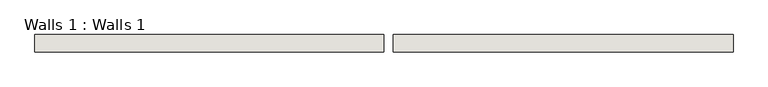
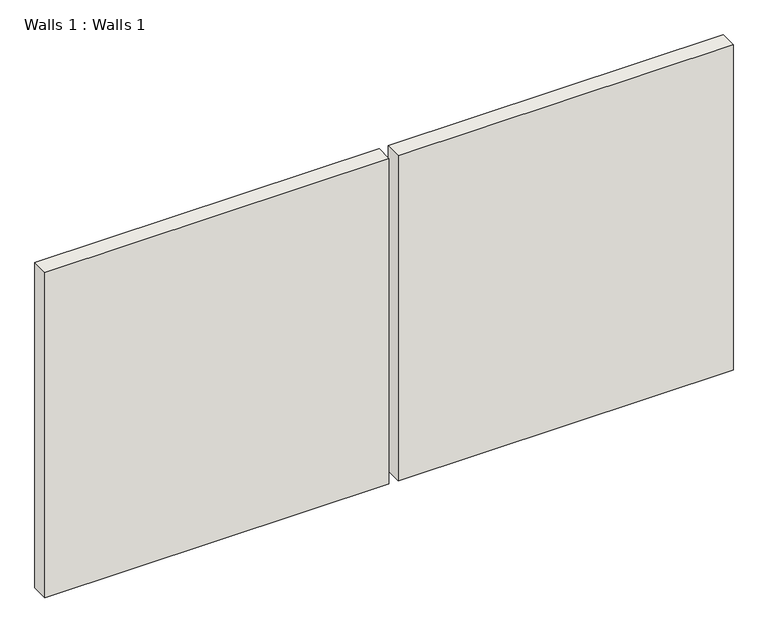
"""IFC4 building model written with IfcOpenShell, lengths in millimetres: wall geometry, Walls 1 : Walls 1."""

from ifc_helpers import new_model, si_unit, origin, origin_with_axes, place, context, project, spatial, polyline, outline, extrude, source, transform, mapped, element, save


def walls_1_walls_1_5f19503e(model_context):
    return source(origin(), model_context, "Body", "SweptSolid", [
        extrude(outline(polyline([(-9840.5692849, -1156.6793133), (-9840.5692849, -1080.4793133), (-8316.5692849, -1080.4793133), (-8316.5692849, -1156.6793133), (-9840.5692849, -1156.6793133)])), origin_with_axes(), (0.0, 0.0, 1.0), 1524.0),
        extrude(outline(polyline([(-6792.5692849, -1080.4793133), (-6792.5692849, -1156.6793133), (-8276.3865159, -1156.6793133), (-8276.3865159, -1080.4793133), (-6792.5692849, -1080.4793133)])), origin_with_axes(), (0.0, 0.0, 1.0), 1524.0),
    ])


if __name__ == "__main__":
    model = new_model("IFC4")
    model_context = context("Model", 3, world=origin())
    ifc_project = project(units=[si_unit("LENGTHUNIT", "METRE", prefix="MILLI")], contexts=[model_context])
    site = spatial("IfcSite", under=ifc_project)
    building = spatial("IfcBuilding", under=site)
    placement = place(None, origin())
    walls_1_walls_1_shape = walls_1_walls_1_5f19503e(model_context)
    element("IfcWall", 1, ObjectType="Walls 1 : Walls 1", at=placement, inside=building, context=model_context, shape_type="MappedRepresentation", body=[
        mapped(walls_1_walls_1_shape, transform((0.0, 0.0, 0.0), x_axis=(1.0, 0.0, 0.0), y_axis=(0.0, 1.0, 0.0), z_axis=(0.0, 0.0, 1.0))),
    ])
    save(model, "model.ifc")

# Revit data of these elements
# Element 1 (IfcWall, "Walls 1 : Walls 1")
#   Materials on its faces: "Metal Deck"
# Materials
#   "Metal Deck": class "Metal", colour RGB 83 83 80, transparency 0, Description = "Steel, mill finish", Cost = 0
